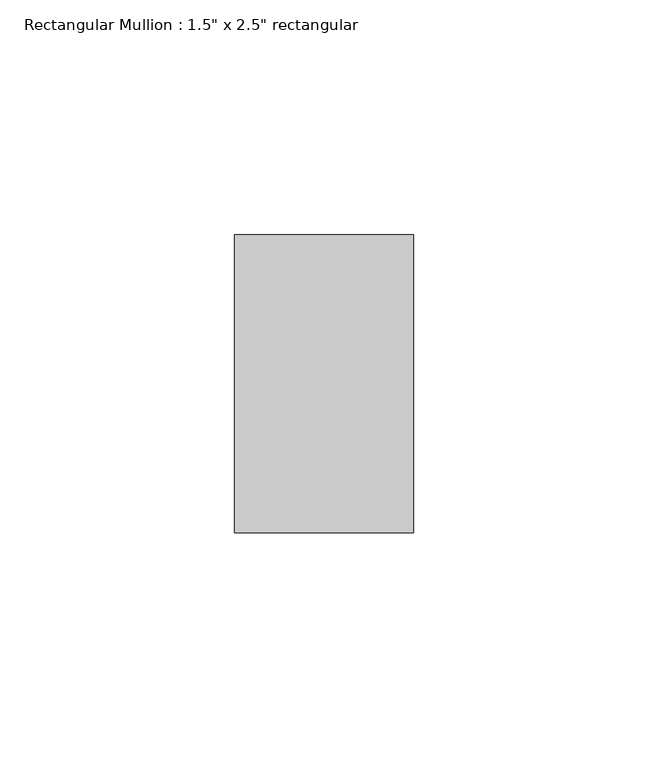
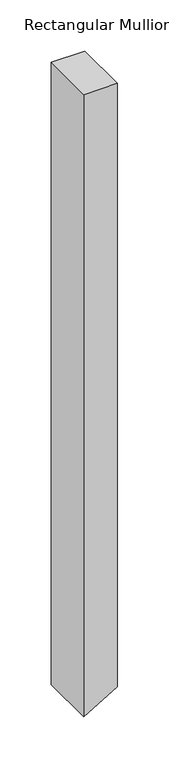
"""IFC4 building model written with IfcOpenShell, lengths in millimetres: member geometry."""

from ifc_helpers import new_model, si_unit, frame, origin, place, context, project, spatial, polyline, outline, extrude, source, transform, mapped, element, save


def member_ee25ef0f(model_context):
    return source(origin(), model_context, "Body", "SweptSolid", [
        extrude(outline(polyline([(0.0, 19.05), (0.0, -19.05), (-742.0054653, -19.05), (-719.3609514, 19.05), (0.0, 19.05)])), frame((0.0, -31.75, 0.0), z_axis=(0.0, 1.0, 0.0), x_axis=(0.0, 0.0, 1.0)), (0.0, 0.0, 1.0), 63.5),
    ])


if __name__ == "__main__":
    model = new_model("IFC4")
    model_context = context("Model", 3, world=origin())
    ifc_project = project(units=[si_unit("LENGTHUNIT", "METRE", prefix="MILLI")], contexts=[model_context])
    site = spatial("IfcSite", under=ifc_project)
    building = spatial("IfcBuilding", under=site)
    placement = place(None, origin())
    member_shape = member_ee25ef0f(model_context)
    element("IfcMember", 1, ObjectType="Rectangular Mullion : 1.5\" x 2.5\" rectangular", at=placement, inside=building, context=model_context, shape_type="MappedRepresentation", body=[
        mapped(member_shape, transform((0.0, 0.0, 0.0), x_axis=(1.0, 0.0, 0.0), y_axis=(0.0, 1.0, 0.0), z_axis=(0.0, 0.0, 1.0))),
    ])
    save(model, "model.ifc")

# Revit data of these elements
# Type "Rectangular Mullion : 1.5\" x 2.5\" rectangular"
#   built-in parameter 1007304 = 0.208333 (stored number, unit not read)
#   built-in parameter 1007301 = 0.0625 (stored number, unit not read)
#   built-in parameter 1007300 = 0.0625 (stored number, unit not read)
